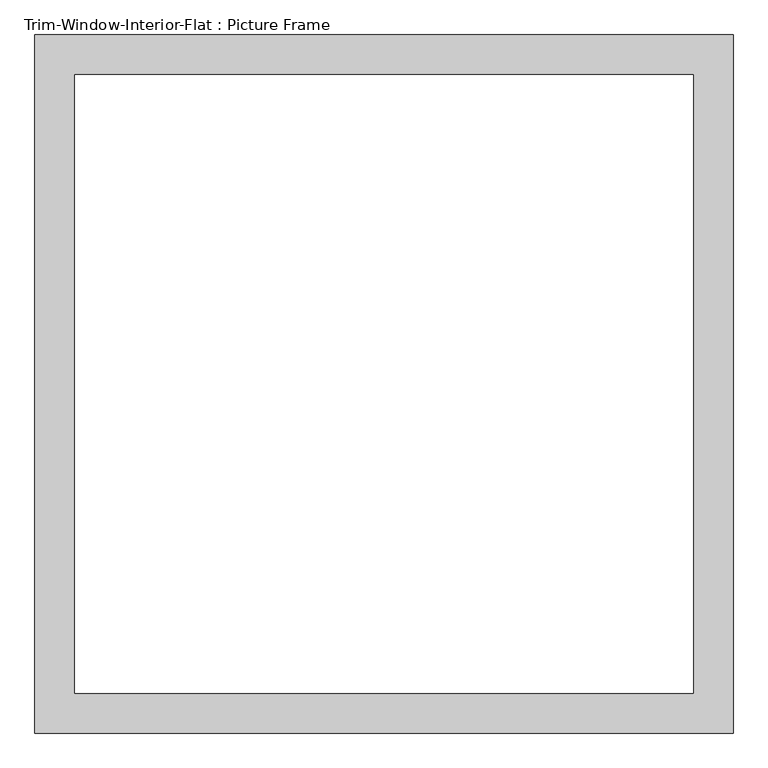
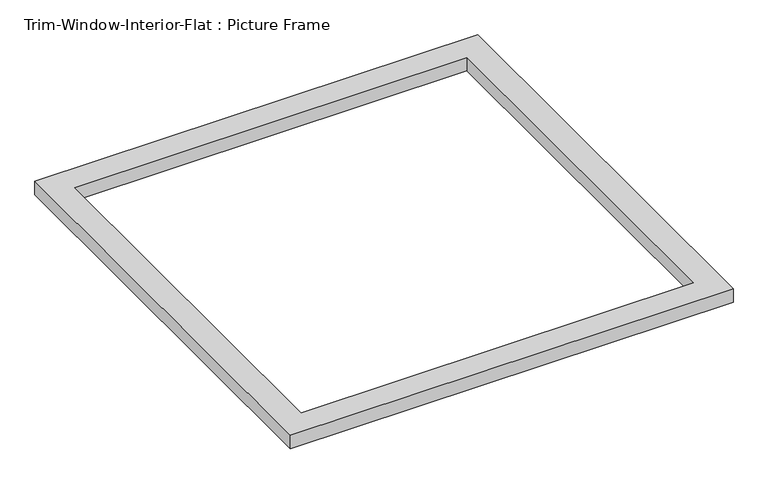
"""IFC4 building model written with IfcOpenShell, lengths in millimetres: proxy geometry, Trim-Window-Interior-Flat : Picture Frame."""

from ifc_helpers import new_model, si_unit, origin, origin_with_axes, place, context, project, spatial, polyline, outline, extrude, source, transform, mapped, element, save


def trim_window_interior_flat_picture_frame_28d4e5dc(model_context):
    return source(origin(), model_context, "Body", "SweptSolid", [
        extrude(outline(polyline([(501.65, 44.45), (501.65, -958.85), (-501.65, -958.85), (-501.65, 44.45), (501.65, 44.45)]), holes=[polyline([(444.5, -12.7), (-444.5, -12.7), (-444.5, -901.7), (444.5, -901.7), (444.5, -12.7)])]), origin_with_axes(), (0.0, 0.0, 1.0), 31.75),
    ])


if __name__ == "__main__":
    model = new_model("IFC4")
    model_context = context("Model", 3, world=origin())
    ifc_project = project(units=[si_unit("LENGTHUNIT", "METRE", prefix="MILLI")], contexts=[model_context])
    site = spatial("IfcSite", under=ifc_project)
    building = spatial("IfcBuilding", under=site)
    placement = place(None, origin())
    trim_window_interior_flat_picture_frame_shape = trim_window_interior_flat_picture_frame_28d4e5dc(model_context)
    element("IfcBuildingElementProxy", 1, Name="Trim-Window-Interior-Flat : Picture Frame", ObjectType="Trim-Window-Interior-Flat : Picture Frame", at=placement, inside=building, context=model_context, shape_type="MappedRepresentation", body=[
        mapped(trim_window_interior_flat_picture_frame_shape, transform((0.0, 0.0, 0.0), x_axis=(1.0, 0.0, 0.0), y_axis=(0.0, 1.0, 0.0), z_axis=(0.0, 0.0, 1.0))),
    ])
    save(model, "model.ifc")

# Revit data of these elements
# Type "Trim-Window-Interior-Flat : Picture Frame"
#   Trim Thickness_Picture Frame = 0' - 1 1/4"
#   Trim Width = 0' - 2 1/4"
#   Trim Thickness_with Sill = 0' - 0 3/4"
#   Sill Thickness = 0' - 1 1/4"
#   Opening Width [instance default] = 2' - 0"
#   Opening Height [instance default] = 3' - 0"
#   Default Elevation = 4' - 0"
#   Sill = no
#   Picture Frame = yes
#   Trim Material [instance default] = none
# Element 1 (IfcBuildingElementProxy, "Trim-Window-Interior-Flat : Picture Frame")
#   Opening Width = 3' - 0"
#   Trim Material = Wood - Stained
#   Materials on its faces: "Wood - Stained"
# Materials
#   "Wood - Stained": class "Wood", colour RGB 227 170 128, transparency 0, Cost = 0
